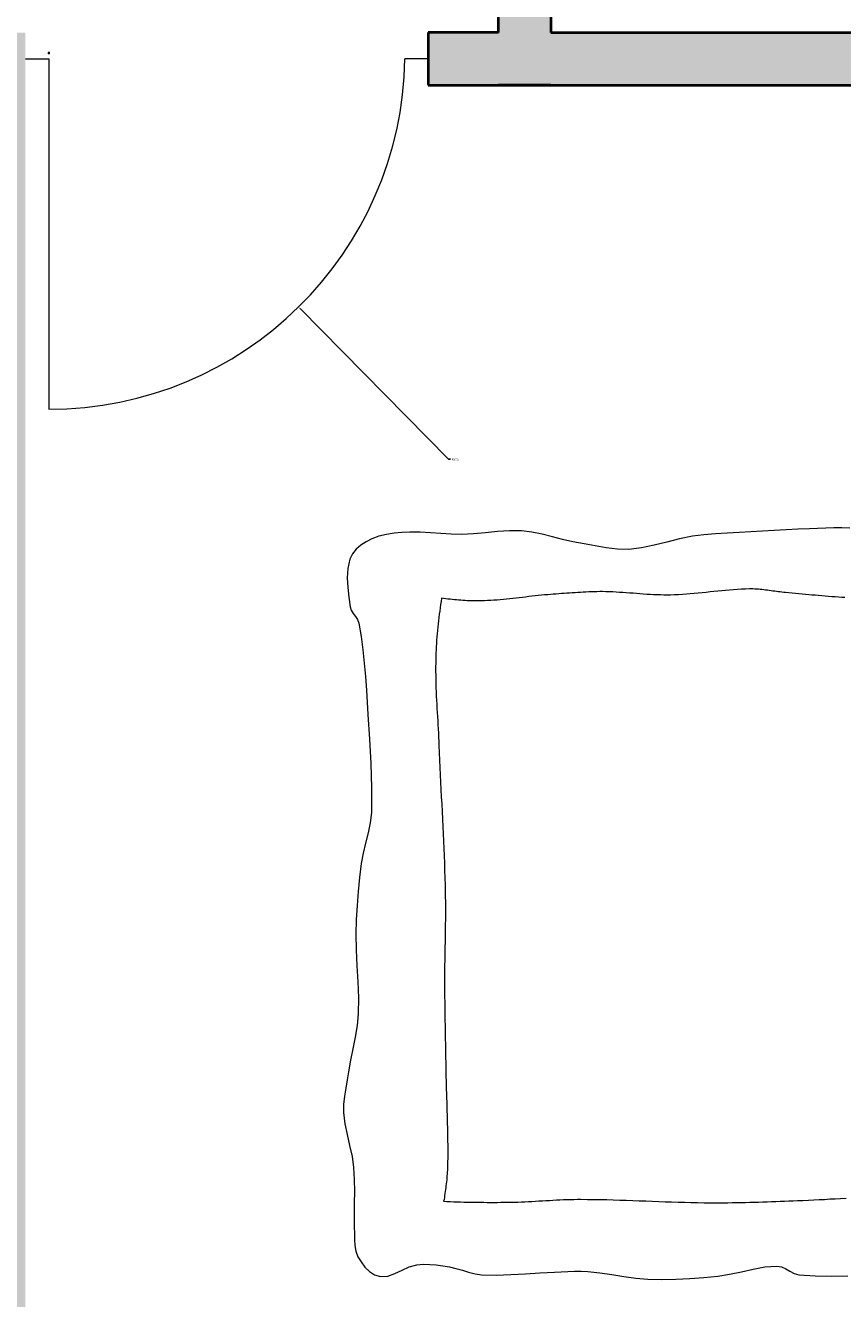
# Model space of a CAD drawing. Units: inches. Extents: x 1441 to 2460, y 1648 to 2683.
# Tile 4 of 35: x 1760 to 1830, y 1866 to 1975. Entities that reach past the tile are written whole.
import ezdxf

# ---------------------------------------------------------------- set-up
doc = ezdxf.new("R2010")
doc.units = ezdxf.units.IN
for name, color, linetype, lineweight in [('A-ANNO-DIMS', 2, 'Continuous', 18), ('A-DOOR', 3, 'Continuous', 20), ('A-FURN', 8, 'Continuous', 15), ('A-WALL', 7, 'Continuous', 40)]:
    doc.layers.add(name, color=color, linetype=linetype, lineweight=lineweight)
doc.layers.add('A-WALL-PATT', color=251, linetype='Continuous', lineweight=13, true_color=0x636466)
doc.styles.get("Standard").update_dxf_attribs({"font": 'arial.ttf'})
doc.dimstyles.get("Standard").update_dxf_attribs({"dimtxt": 0.18, "dimasz": 0.18, "dimexe": 0.18, "dimexo": 0.0625, "dimgap": 0.09, "dimtad": 0, "dimtih": 1, "dimtoh": 1, "dimdec": 4, "dimzin": 0, "dimdsep": 46, "dimtxsty": 'Standard', "dimcen": 0.09, "dimadec": 0, "dimazin": 0, "dimtfac": 1, "dimtdec": 4, "dimtofl": 0, "dimtmove": 0, "dimatfit": 3, "dimfxl": 1, "dimtolj": 1, "dimtzin": 0, "dimarcsym": 0})

# ---------------------------------------------------------------- blocks, each defined once
blk = doc.blocks.new('BED-DOUBLE-PLAN')
for p, q in [((0.03, 43.36), (0, 42.67)), ((0, 42.67), (0, 41.98)), ((5.96, 42.66), (5.93, 42.38)), ((5.97, 42.94), (5.96, 42.66)), ((57.42, 42.57), (57.39, 43.03)), ((57.45, 42.11), (57.42, 42.57)), ((64.07, 41.78), (64.06, 43.17)), ((0, 41.98), (0.02, 41.29)), ((5.87, 41.53), (5.85, 41.24)), ((5.89, 41.81), (5.87, 41.53)), ((5.91, 42.09), (5.89, 41.81)), ((5.93, 42.38), (5.91, 42.09)), ((57.47, 41.65), (57.45, 42.11)), ((57.5, 41.19), (57.47, 41.65)), ((64.05, 40.38), (64.07, 41.78)), ((0.02, 41.29), (0.05, 40.6)), ((0.05, 40.6), (0.08, 39.91)), ((5.77, 40.39), (5.75, 40.11)), ((5.8, 40.68), (5.77, 40.39)), ((5.82, 40.96), (5.8, 40.68)), ((5.85, 41.24), (5.82, 40.96)), ((57.52, 40.73), (57.5, 41.19)), ((57.55, 40.27), (57.52, 40.73)), ((63.96, 38.99), (64.05, 40.38)), ((0.08, 39.91), (0.12, 38.9)), ((5.67, 39.26), (5.65, 38.98)), ((5.7, 39.55), (5.67, 39.26)), ((5.72, 39.83), (5.7, 39.55)), ((5.75, 40.11), (5.72, 39.83)), ((57.57, 39.81), (57.55, 40.27)), ((57.59, 39.34), (57.57, 39.81)), ((57.61, 38.88), (57.59, 39.34)), ((0.12, 38.9), (0.17, 37.89)), ((5.6, 38.41), (5.57, 38.13)), ((5.62, 38.7), (5.6, 38.41)), ((5.65, 38.98), (5.62, 38.7)), ((57.62, 38.51), (57.61, 38.88)), ((57.64, 38.14), (57.62, 38.51)), ((63.45, 37.87), (63.66, 38.23)), ((63.66, 38.23), (63.85, 38.6)), ((63.85, 38.6), (63.96, 38.99)), ((0.17, 37.89), (0.23, 36.88)), ((5.45, 37.07), (5.43, 36.92)), ((5.47, 37.23), (5.45, 37.07)), ((5.49, 37.38), (5.47, 37.23)), ((5.51, 37.54), (5.49, 37.38)), ((5.53, 37.69), (5.51, 37.54)), ((5.54, 37.85), (5.53, 37.69)), ((5.57, 38.13), (5.54, 37.85)), ((57.65, 37.77), (57.64, 38.14)), ((57.67, 37.39), (57.65, 37.77)), ((57.68, 37.02), (57.67, 37.39)), ((63.21, 37.11), (63.27, 37.5)), ((63.29, 36.09), (63.21, 37.11)), ((63.27, 37.5), (63.45, 37.87)), ((0.23, 36.88), (0.29, 35.88)), ((5.3, 35.99), (5.29, 35.83)), ((5.32, 36.14), (5.3, 35.99)), ((5.34, 36.3), (5.32, 36.14)), ((5.37, 36.45), (5.34, 36.3)), ((5.39, 36.61), (5.37, 36.45)), ((5.41, 36.76), (5.39, 36.61)), ((5.43, 36.92), (5.41, 36.76)), ((57.69, 36.65), (57.68, 37.02)), ((57.71, 36.27), (57.69, 36.65)), ((57.72, 35.9), (57.71, 36.27)), ((63.47, 35.08), (63.29, 36.09)), ((0.29, 35.88), (0.35, 34.87)), ((5.24, 35.21), (5.23, 35.06)), ((5.23, 35.06), (5.23, 34.9)), ((5.23, 34.9), (5.23, 34.75)), ((5.26, 35.52), (5.24, 35.37)), ((5.24, 35.37), (5.24, 35.21)), ((5.27, 35.68), (5.26, 35.52)), ((5.29, 35.83), (5.27, 35.68)), ((57.73, 35.53), (57.72, 35.9)), ((57.74, 35.15), (57.73, 35.53)), ((57.75, 34.78), (57.74, 35.15)), ((63.7, 34.07), (63.47, 35.08)), ((0.35, 34.87), (0.4, 33.87)), ((0.4, 33.87), (0.46, 32.86)), ((5.23, 34.75), (5.24, 34.41)), ((5.24, 34.41), (5.25, 34.07)), ((5.25, 34.07), (5.27, 33.73)), ((57.76, 34.41), (57.75, 34.78)), ((57.77, 34.04), (57.76, 34.41)), ((57.78, 33.66), (57.77, 34.04)), ((63.92, 33.06), (63.7, 34.07)), ((0.46, 32.86), (0.52, 31.86)), ((5.27, 33.73), (5.3, 33.4)), ((5.3, 33.4), (5.32, 33.06)), ((5.32, 33.06), (5.35, 32.72)), ((5.35, 32.72), (5.39, 32.39)), ((57.78, 33.29), (57.78, 33.66)), ((57.79, 32.92), (57.78, 33.29)), ((57.79, 32.54), (57.79, 32.92)), ((64.08, 32.05), (63.92, 33.06)), ((0.52, 31.86), (0.6, 30.86)), ((5.39, 32.39), (5.42, 32.05)), ((5.42, 32.05), (5.46, 31.71)), ((5.46, 31.71), (5.49, 31.38)), ((57.79, 32.17), (57.79, 32.54)), ((57.79, 31.8), (57.79, 32.17)), ((57.79, 31.42), (57.79, 31.8)), ((64.19, 30.85), (64.08, 32.05)), ((0.6, 30.86), (0.72, 29.87)), ((5.49, 31.38), (5.53, 31.04)), ((5.53, 31.04), (5.56, 30.7)), ((5.56, 30.7), (5.59, 30.37)), ((57.78, 30.31), (57.79, 30.87)), ((57.79, 30.87), (57.79, 31.42)), ((64.27, 29.65), (64.19, 30.85)), ((0.72, 29.87), (0.93, 28.77)), ((5.59, 30.37), (5.63, 30.03)), ((5.63, 30.03), (5.66, 29.69)), ((5.66, 29.69), (5.68, 29.36)), ((57.75, 29.2), (57.77, 29.76)), ((57.77, 29.76), (57.78, 30.31)), ((64.33, 28.45), (64.27, 29.65)), ((0.93, 28.77), (1.21, 27.69)), ((5.68, 29.36), (5.71, 29.02)), ((5.71, 29.02), (5.73, 28.68)), ((5.73, 28.68), (5.74, 28.34)), ((57.72, 28.09), (57.74, 28.65)), ((57.74, 28.65), (57.75, 29.2)), ((64.35, 27.25), (64.33, 28.45)), ((1.21, 27.69), (1.49, 26.61)), ((5.74, 28.34), (5.75, 28.01)), ((5.75, 27.42), (5.74, 27.13)), ((5.75, 28.01), (5.75, 27.71)), ((5.75, 27.71), (5.75, 27.42)), ((57.68, 26.99), (57.7, 27.54)), ((57.7, 27.54), (57.72, 28.09)), ((1.49, 26.61), (1.72, 25.52)), ((5.7, 26.26), (5.69, 25.96)), ((5.72, 26.55), (5.7, 26.26)), ((5.73, 26.84), (5.72, 26.55)), ((5.74, 27.13), (5.73, 26.84)), ((57.64, 25.88), (57.66, 26.43)), ((57.66, 26.43), (57.68, 26.99)), ((64.33, 26.05), (64.35, 27.25)), ((1.72, 25.52), (1.85, 24.42)), ((5.62, 25.09), (5.6, 24.8)), ((5.64, 25.38), (5.62, 25.09)), ((5.67, 25.67), (5.64, 25.38)), ((5.69, 25.96), (5.67, 25.67)), ((57.59, 24.77), (57.62, 25.32)), ((57.62, 25.32), (57.64, 25.88)), ((64.25, 25.02), (64.33, 26.05)), ((1.85, 24.42), (1.83, 23.46)), ((5.56, 24.21), (5.54, 23.92)), ((5.58, 24.51), (5.56, 24.21)), ((5.6, 24.8), (5.58, 24.51)), ((57.56, 23.66), (57.57, 24.21)), ((57.57, 24.21), (57.59, 24.77)), ((63.94, 22.97), (64.11, 23.99)), ((64.11, 23.99), (64.25, 25.02)), ((1.83, 23.46), (1.72, 22.5)), ((5.49, 23.05), (5.47, 22.75)), ((5.5, 23.34), (5.49, 23.05)), ((5.52, 23.63), (5.5, 23.34)), ((5.54, 23.92), (5.52, 23.63)), ((57.52, 22.55), (57.54, 23.1)), ((57.54, 23.1), (57.56, 23.66)), ((63.78, 21.94), (63.94, 22.97)), ((1.72, 22.5), (1.55, 21.54)), ((5.47, 22.46), (5.46, 22.17)), ((5.46, 22.17), (5.46, 21.94)), ((5.46, 21.94), (5.47, 21.7)), ((5.47, 22.75), (5.47, 22.46)), ((57.5, 21.44), (57.51, 21.99)), ((57.51, 21.99), (57.52, 22.55)), ((63.67, 20.91), (63.78, 21.94)), ((1.55, 21.54), (1.36, 20.59)), ((5.47, 21.7), (5.47, 21.47)), ((5.47, 21.47), (5.48, 21.23)), ((5.48, 21.23), (5.49, 21)), ((5.49, 21), (5.5, 20.76)), ((5.5, 20.76), (5.51, 20.53)), ((57.49, 20.33), (57.5, 20.88)), ((57.5, 20.88), (57.5, 21.44)), ((63.65, 20.35), (63.67, 20.91)), ((1.18, 19.64), (1, 18.76)), ((1.36, 20.59), (1.18, 19.64)), ((5.51, 20.53), (5.52, 20.29)), ((5.52, 20.29), (5.53, 20.06)), ((5.53, 20.06), (5.55, 19.83)), ((5.55, 19.83), (5.56, 19.59)), ((57.49, 20.03), (57.49, 20.33)), ((57.5, 19.73), (57.49, 20.03)), ((57.5, 19.43), (57.5, 19.73)), ((63.66, 19.78), (63.65, 20.35)), ((63.68, 19.21), (63.66, 19.78)), ((1, 18.76), (0.77, 17.89)), ((5.56, 19.59), (5.58, 19.36)), ((5.58, 19.36), (5.59, 19.12)), ((5.59, 19.12), (5.61, 18.89)), ((5.61, 18.89), (5.63, 18.66)), ((5.63, 18.66), (5.65, 18.42)), ((57.51, 19.13), (57.5, 19.43)), ((57.52, 18.83), (57.51, 19.13)), ((57.54, 18.53), (57.52, 18.83)), ((63.71, 18.64), (63.68, 19.21)), ((63.74, 18.07), (63.71, 18.64)), ((0.77, 17.89), (0.55, 17.01)), ((5.65, 18.42), (5.67, 18.19)), ((5.67, 18.19), (5.68, 17.95)), ((5.68, 17.95), (5.7, 17.72)), ((5.7, 17.72), (5.72, 17.49)), ((5.72, 17.49), (5.74, 17.21)), ((57.55, 18.23), (57.54, 18.53)), ((57.57, 17.93), (57.55, 18.23)), ((57.59, 17.63), (57.57, 17.93)), ((57.6, 17.33), (57.59, 17.63)), ((63.8, 16.82), (63.74, 18.07)), ((0.55, 17.01), (0.37, 16.13)), ((5.74, 17.21), (5.77, 16.94)), ((5.77, 16.94), (5.79, 16.67)), ((5.79, 16.67), (5.82, 16.4)), ((5.82, 16.4), (5.85, 16.13)), ((57.62, 17.03), (57.6, 17.33)), ((57.64, 16.73), (57.62, 17.03)), ((57.66, 16.43), (57.64, 16.73)), ((57.68, 16.13), (57.66, 16.43)), ((63.88, 15.57), (63.8, 16.82)), ((0.37, 16.13), (0.26, 15.25)), ((5.85, 16.13), (5.88, 15.86)), ((5.88, 15.86), (5.92, 15.59)), ((5.92, 15.59), (5.95, 15.32)), ((5.95, 15.32), (5.98, 15.04)), ((57.69, 15.83), (57.68, 16.13)), ((57.71, 15.53), (57.69, 15.83)), ((57.72, 15.23), (57.71, 15.53)), ((63.95, 14.32), (63.88, 15.57)), ((0.26, 15.25), (0.24, 14.22)), ((0.24, 14.22), (0.31, 13.19)), ((5.98, 15.04), (6.01, 14.77)), ((6.01, 14.77), (6.04, 14.5)), ((6.04, 14.5), (6.07, 14.23)), ((6.07, 14.23), (6.1, 13.96)), ((57.73, 14.93), (57.72, 15.23)), ((57.74, 14.63), (57.73, 14.93)), ((57.74, 14.33), (57.74, 14.63)), ((57.75, 14.04), (57.74, 14.33)), ((63.99, 13.07), (63.95, 14.32)), ((0.31, 13.19), (0.41, 12.16)), ((6.1, 13.96), (6.13, 13.69)), ((6.13, 13.69), (6.16, 13.42)), ((6.16, 13.42), (6.18, 13.15)), ((6.18, 13.15), (6.2, 12.88)), ((57.75, 13.75), (57.75, 14.04)), ((57.75, 13.46), (57.75, 13.75)), ((57.76, 13.17), (57.75, 13.46)), ((57.76, 12.89), (57.76, 13.17)), ((0.41, 12.16), (0.51, 11.13)), ((6.2, 12.88), (6.22, 12.6)), ((6.22, 12.6), (6.23, 12.33)), ((6.23, 12.33), (6.24, 12.06)), ((6.24, 12.06), (6.25, 11.88)), ((57.75, 12.02), (57.76, 12.31)), ((57.75, 11.73), (57.75, 12.02)), ((57.76, 12.6), (57.76, 12.89)), ((57.76, 12.31), (57.76, 12.6)), ((63.96, 11.82), (63.99, 13.07)), ((0.51, 11.13), (0.56, 10.1)), ((6.25, 10.96), (6.24, 10.77)), ((6.25, 11.88), (6.25, 11.69)), ((6.25, 11.69), (6.25, 11.51)), ((6.25, 11.51), (6.25, 11.32)), ((6.25, 11.32), (6.25, 11.14)), ((6.25, 11.14), (6.25, 10.96)), ((57.74, 11.16), (57.75, 11.45)), ((57.74, 10.87), (57.74, 11.16)), ((57.75, 11.45), (57.75, 11.73)), ((63.75, 10.71), (63.89, 11.26)), ((63.89, 11.26), (63.96, 11.82)), ((0.56, 10.1), (0.54, 9.21)), ((6.19, 9.85), (6.17, 9.67)), ((6.2, 10.04), (6.19, 9.85)), ((6.22, 10.22), (6.2, 10.04)), ((6.23, 10.4), (6.22, 10.22)), ((6.24, 10.59), (6.23, 10.4)), ((6.24, 10.77), (6.24, 10.59)), ((57.71, 9.72), (57.72, 10.01)), ((57.72, 10.01), (57.73, 10.29)), ((57.73, 10.58), (57.74, 10.87)), ((57.73, 10.29), (57.73, 10.58)), ((63.41, 9.62), (63.57, 10.17)), ((63.57, 10.17), (63.75, 10.71)), ((0.54, 9.21), (0.48, 8.33)), ((6.07, 8.76), (6.04, 8.57)), ((6.09, 8.94), (6.07, 8.76)), ((6.11, 9.12), (6.09, 8.94)), ((6.14, 9.3), (6.11, 9.12)), ((6.16, 9.49), (6.14, 9.3)), ((6.17, 9.67), (6.16, 9.49)), ((44.18, 8.72), (44.58, 8.72)), ((44.58, 8.72), (44.98, 8.73)), ((44.98, 8.73), (45.38, 8.74)), ((45.38, 8.74), (45.77, 8.75)), ((45.77, 8.75), (46.17, 8.75)), ((46.17, 8.75), (46.57, 8.76)), ((46.57, 8.76), (46.97, 8.77)), ((46.97, 8.77), (47.34, 8.78)), ((47.34, 8.78), (47.7, 8.78)), ((47.7, 8.78), (48.07, 8.79)), ((48.07, 8.79), (48.44, 8.8)), ((48.44, 8.8), (48.81, 8.82)), ((48.81, 8.82), (49.17, 8.83)), ((49.17, 8.83), (49.54, 8.84)), ((49.54, 8.84), (49.91, 8.85)), ((49.91, 8.85), (50.28, 8.86)), ((50.28, 8.86), (50.65, 8.87)), ((50.65, 8.87), (51.01, 8.88)), ((51.01, 8.88), (51.38, 8.89)), ((51.38, 8.89), (51.75, 8.9)), ((51.75, 8.9), (52.12, 8.91)), ((52.12, 8.91), (52.48, 8.91)), ((52.48, 8.91), (52.85, 8.92)), ((52.85, 8.92), (53.22, 8.92)), ((53.22, 8.92), (53.59, 8.92)), ((53.59, 8.92), (53.95, 8.92)), ((53.95, 8.92), (54.32, 8.91)), ((54.32, 8.91), (54.49, 8.91)), ((54.49, 8.91), (54.66, 8.9)), ((54.66, 8.9), (54.83, 8.9)), ((54.83, 8.9), (55, 8.89)), ((55, 8.89), (55.16, 8.88)), ((55.16, 8.88), (55.33, 8.87)), ((55.33, 8.87), (55.5, 8.85)), ((55.5, 8.85), (55.67, 8.84)), ((55.67, 8.84), (55.84, 8.83)), ((55.84, 8.83), (56, 8.81)), ((56, 8.81), (56.17, 8.79)), ((56.17, 8.79), (56.34, 8.77)), ((56.34, 8.77), (56.51, 8.75)), ((56.51, 8.75), (56.67, 8.73)), ((56.67, 8.73), (56.84, 8.71)), ((57.67, 8.57), (57.68, 8.85)), ((57.68, 8.85), (57.69, 9.14)), ((57.69, 9.14), (57.7, 9.43)), ((57.7, 9.43), (57.71, 9.72)), ((63.2, 8.51), (63.28, 9.07)), ((63.28, 9.07), (63.41, 9.62)), ((0.48, 8.33), (0.41, 7.44)), ((6.04, 8.57), (6.01, 8.39)), ((6.01, 8.39), (6.29, 8.35)), ((6.29, 8.35), (6.56, 8.31)), ((6.56, 8.31), (6.84, 8.27)), ((6.84, 8.27), (7.12, 8.23)), ((7.12, 8.23), (7.39, 8.19)), ((7.39, 8.19), (7.67, 8.16)), ((7.67, 8.16), (7.95, 8.12)), ((7.95, 8.12), (8.23, 8.09)), ((8.23, 8.09), (8.5, 8.07)), ((8.5, 8.07), (8.78, 8.04)), ((8.78, 8.04), (9.06, 8.02)), ((9.06, 8.02), (9.34, 7.99)), ((9.34, 7.99), (9.62, 7.97)), ((9.62, 7.97), (9.9, 7.95)), ((9.9, 7.95), (10.18, 7.94)), ((10.18, 7.94), (10.45, 7.92)), ((10.45, 7.92), (10.73, 7.91)), ((10.73, 7.91), (11.01, 7.9)), ((11.01, 7.9), (11.29, 7.89)), ((11.29, 7.89), (11.57, 7.89)), ((11.57, 7.89), (11.92, 7.88)), ((11.92, 7.88), (12.28, 7.88)), ((12.28, 7.88), (12.63, 7.89)), ((12.63, 7.89), (12.98, 7.89)), ((12.98, 7.89), (13.34, 7.9)), ((13.34, 7.9), (13.69, 7.91)), ((13.69, 7.91), (14.04, 7.92)), ((14.04, 7.92), (14.4, 7.94)), ((14.4, 7.94), (14.75, 7.96)), ((14.75, 7.96), (15.1, 7.98)), ((15.1, 7.98), (15.46, 7.99)), ((15.46, 7.99), (15.81, 8.01)), ((15.81, 8.01), (16.16, 8.04)), ((16.16, 8.04), (16.52, 8.06)), ((16.52, 8.06), (16.87, 8.08)), ((16.87, 8.08), (17.22, 8.1)), ((17.22, 8.1), (17.58, 8.12)), ((17.58, 8.12), (17.93, 8.13)), ((17.93, 8.13), (18.28, 8.15)), ((18.28, 8.15), (18.64, 8.17)), ((18.64, 8.17), (19.27, 8.19)), ((19.27, 8.19), (19.9, 8.22)), ((19.9, 8.22), (20.52, 8.25)), ((20.52, 8.25), (21.15, 8.28)), ((21.15, 8.28), (21.78, 8.31)), ((21.78, 8.31), (22.41, 8.34)), ((22.41, 8.34), (23.04, 8.37)), ((23.04, 8.37), (23.67, 8.4)), ((23.67, 8.4), (24.3, 8.43)), ((24.3, 8.43), (24.93, 8.46)), ((24.93, 8.46), (25.56, 8.49)), ((25.56, 8.49), (26.19, 8.52)), ((26.19, 8.52), (26.82, 8.55)), ((26.82, 8.55), (27.45, 8.58)), ((27.45, 8.58), (28.08, 8.6)), ((28.08, 8.6), (28.71, 8.63)), ((28.71, 8.63), (29.33, 8.65)), ((29.33, 8.65), (29.96, 8.67)), ((29.96, 8.67), (30.59, 8.69)), ((30.59, 8.69), (31.22, 8.7)), ((31.22, 8.7), (31.61, 8.71)), ((31.61, 8.71), (32, 8.72)), ((32, 8.72), (32.39, 8.72)), ((32.39, 8.72), (32.78, 8.72)), ((32.78, 8.72), (33.17, 8.72)), ((33.17, 8.72), (33.56, 8.72)), ((33.56, 8.72), (33.95, 8.71)), ((33.95, 8.71), (34.34, 8.71)), ((34.34, 8.71), (34.73, 8.7)), ((34.73, 8.7), (35.12, 8.69)), ((35.12, 8.69), (35.51, 8.69)), ((35.51, 8.69), (35.89, 8.68)), ((35.89, 8.68), (36.28, 8.67)), ((36.28, 8.67), (36.67, 8.67)), ((36.67, 8.67), (37.06, 8.66)), ((37.06, 8.66), (37.45, 8.65)), ((37.45, 8.65), (37.84, 8.65)), ((37.84, 8.65), (38.23, 8.65)), ((38.23, 8.65), (38.62, 8.64)), ((38.62, 8.64), (39.01, 8.65)), ((39.01, 8.65), (39.41, 8.65)), ((39.41, 8.65), (39.81, 8.65)), ((39.81, 8.65), (40.2, 8.65)), ((40.2, 8.65), (40.6, 8.66)), ((40.6, 8.66), (41, 8.66)), ((41, 8.66), (41.4, 8.67)), ((41.4, 8.67), (41.8, 8.67)), ((41.8, 8.67), (42.19, 8.68)), ((42.19, 8.68), (42.59, 8.69)), ((42.59, 8.69), (42.99, 8.69)), ((42.99, 8.69), (43.39, 8.7)), ((43.39, 8.7), (43.78, 8.71)), ((43.78, 8.71), (44.18, 8.72)), ((56.84, 8.71), (57.01, 8.68)), ((57.01, 8.68), (57.17, 8.65)), ((57.17, 8.65), (57.34, 8.63)), ((57.34, 8.63), (57.51, 8.6)), ((57.51, 8.6), (57.67, 8.57)), ((63.07, 7.38), (63.12, 7.94)), ((63.12, 7.94), (63.2, 8.51)), ((0.41, 7.44), (0.36, 6.56)), ((0.36, 6.56), (0.37, 5.67)), ((63.06, 6.82), (63.07, 7.38)), ((63.1, 6.26), (63.06, 6.82)), ((0.37, 5.67), (0.4, 5)), ((63.28, 5.62), (63.1, 6.26)), ((63.56, 5.01), (63.28, 5.62)), ((0.4, 5), (0.46, 4.34)), ((63.86, 4.4), (63.56, 5.01)), ((64.07, 3.78), (63.86, 4.4)), ((0.46, 4.34), (0.56, 3.68)), ((0.56, 3.68), (0.71, 3.03)), ((64.1, 3.15), (64.07, 3.78)), ((0.71, 3.03), (0.94, 2.41)), ((0.94, 2.41), (1.18, 1.94)), ((15.99, 2.09), (18.08, 2.23)), ((18.08, 2.23), (20.17, 2.34)), ((20.17, 2.34), (22.27, 2.4)), ((22.27, 2.4), (24.37, 2.38)), ((24.37, 2.38), (25.25, 2.29)), ((25.25, 2.29), (26.12, 2.11)), ((63.3, 1.83), (63.67, 2.22)), ((63.67, 2.22), (63.96, 2.66)), ((63.96, 2.66), (64.1, 3.15)), ((1.18, 1.94), (1.48, 1.49)), ((1.48, 1.49), (1.83, 1.09)), ((7.58, 1.03), (7.85, 1.2)), ((7.85, 1.2), (8.15, 1.31)), ((8.15, 1.31), (9.29, 1.5)), ((9.29, 1.5), (10.43, 1.66)), ((10.43, 1.66), (11.58, 1.77)), ((11.58, 1.77), (12.74, 1.87)), ((12.74, 1.87), (13.89, 1.95)), ((13.89, 1.95), (15.99, 2.09)), ((26.12, 2.11), (26.99, 1.88)), ((26.99, 1.88), (27.86, 1.67)), ((27.86, 1.67), (28.74, 1.51)), ((28.74, 1.51), (29.94, 1.37)), ((29.94, 1.37), (31.14, 1.25)), ((31.14, 1.25), (32.35, 1.16)), ((32.35, 1.16), (33.55, 1.09)), ((36.13, 1.07), (37.5, 1.14)), ((37.5, 1.14), (38.87, 1.22)), ((38.87, 1.22), (40.25, 1.28)), ((40.25, 1.28), (41.62, 1.25)), ((41.62, 1.25), (42.61, 1.16)), ((42.61, 1.16), (43.61, 0.99)), ((61.94, 1.05), (62.41, 1.23)), ((62.41, 1.23), (62.86, 1.5)), ((62.86, 1.5), (63.3, 1.83)), ((1.83, 1.09), (2.23, 0.76)), ((2.23, 0.76), (2.69, 0.54)), ((2.69, 0.54), (3.48, 0.36)), ((3.48, 0.36), (4.29, 0.31)), ((4.29, 0.31), (5.11, 0.35)), ((5.11, 0.35), (5.93, 0.45)), ((5.93, 0.45), (6.75, 0.56)), ((6.75, 0.56), (7.04, 0.66)), ((7.04, 0.66), (7.32, 0.83)), ((7.32, 0.83), (7.58, 1.03)), ((33.55, 1.09), (34.76, 1.05)), ((34.76, 1.05), (36.13, 1.07)), ((43.61, 0.99), (44.6, 0.79)), ((44.6, 0.79), (45.58, 0.59)), ((45.58, 0.59), (46.58, 0.41)), ((46.58, 0.41), (47.27, 0.3)), ((47.27, 0.3), (47.97, 0.18)), ((47.97, 0.18), (48.67, 0.07)), ((48.67, 0.07), (49.37, 0)), ((49.37, 0), (50.07, 0)), ((50.07, 0), (51.02, 0.11)), ((51.02, 0.11), (51.96, 0.3)), ((51.96, 0.3), (52.89, 0.52)), ((52.89, 0.52), (53.83, 0.73)), ((53.83, 0.73), (54.78, 0.86)), ((54.78, 0.86), (55.8, 0.92)), ((55.8, 0.92), (56.82, 0.93)), ((56.82, 0.93), (57.84, 0.91)), ((57.84, 0.91), (58.87, 0.9)), ((58.87, 0.9), (59.89, 0.92)), ((59.89, 0.92), (60.41, 0.93)), ((60.41, 0.93), (60.93, 0.93)), ((60.93, 0.93), (61.44, 0.96)), ((61.44, 0.96), (61.94, 1.05))]:
    blk.add_line(p, q)
blk = doc.blocks.new('DOOR-BED3-30')
for p, q in [((0, 30.01), (2, 30.01)), ((2, 30.01), (2, 0.01)), ((34.49, 30.01), (32.49, 30.01))]:
    blk.add_line(p, q)
blk.add_arc((2, 30.51), 30.5, 270, 359.0598)
blk = doc.blocks.new('*D67')
at = {"layer": 'A-ANNO-DIMS', "color": 0, "lineweight": -2, "transparency": 16777216}
for p, q in [((1889.45, 2298.7), (1916.22, 2298.7)), ((1916.04, 2298.52), (1916.04, 2055.94)), ((1916.04, 1813), (1916.04, 2055.57)), ((1758.22, 1812.82), (1916.22, 1812.82))]:
    blk.add_line(p, q, dxfattribs=at)
at = {"layer": 'A-ANNO-DIMS', "color": 0, "transparency": 16777216}
for points in [[(1916.01, 2298.52), (1916.07, 2298.52), (1916.04, 2298.7)], [(1916.01, 1813), (1916.07, 1813), (1916.04, 1812.82)]]:
    blk.add_solid(points, dxfattribs=at)
at = {"layer": 'Defpoints', "color": 0, "transparency": 16777216}
for p in [(1889.39, 2298.7), (1916.04, 2298.7), (1758.16, 1812.82)]:
    blk.add_point(p, dxfattribs=at)
at = {"layer": 'A-ANNO-DIMS', "color": 0, "transparency": 16777216, "insert": (1916.04, 2055.76), "char_height": 0.18, "attachment_point": 5}
blk.add_mtext('\\A1;485.9', dxfattribs=at)
blk = doc.blocks.new('*D131')
at = {"layer": 'A-ANNO-DIMS', "color": 0, "lineweight": -2, "transparency": 16777216}
for p, q in [((1762.3, 1972.95), (1762.48, 1972.95)), ((1762.39, 1972.86), (1762.39, 1973.04)), ((1796.61, 1938.16), (1783.9, 1951.07)), ((1796.79, 1938.16), (1796.61, 1938.16))]:
    blk.add_line(p, q, dxfattribs=at)
at = {"layer": 'A-ANNO-DIMS', "color": 0, "transparency": 16777216}
blk.add_solid([(1783.92, 1951.09), (1783.88, 1951.05), (1783.77, 1951.2)], dxfattribs=at)
at = {"layer": 'Defpoints', "color": 0, "transparency": 16777216}
for p in [(1762.39, 1972.95), (1783.77, 1951.2)]:
    blk.add_point(p, dxfattribs=at)
at = {"layer": 'A-ANNO-DIMS', "color": 0, "transparency": 16777216, "insert": (1797.2, 1938.16), "char_height": 0.18, "attachment_point": 5}
blk.add_mtext('\\A1;R30.5', dxfattribs=at)

msp = doc.modelspace()

# ---------------------------------------------------------------- hatches: boundary and pattern name
at = {"layer": 'A-WALL-PATT'}
h = msp.add_hatch(color=256, dxfattribs=at)
h.dxf.hatch_style = 1
h.paths.add_polyline_path([(1627.5085, 2298.6952), (1568.8859, 2298.6952), (1568.8859, 2246.9605), (1577.8859, 2246.9605), (1577.8859, 2289.6952), (1627.5085, 2289.6952), (1627.5085, 2294.1952)])
h.paths.add_polyline_path([(1675.5777, 2298.6952), (1651.5085, 2298.6952), (1651.5085, 2289.6952), (1675.5777, 2289.6952), (1675.5777, 2294.1952)])
h.paths.add_polyline_path([(1667.3859, 2289.6952), (1662.8859, 2289.6952), (1662.8859, 2233.0622), (1667.3859, 2233.0622)])
h.paths.add_polyline_path([(1715.8721, 2294.3362), (1715.8721, 2295.2788), (1715.8721, 2298.6952), (1699.5777, 2298.6952), (1699.5777, 2289.6952), (1715.8721, 2289.6952)])
h.paths.add_polyline_path([(1707.8859, 2289.6952), (1703.3859, 2289.6952), (1703.3859, 2199.6952), (1707.8859, 2199.6952)])
h.paths.add_polyline_path([(1760.3859, 2204.637), (1755.8859, 2204.637), (1755.8859, 2199.6952), (1667.3859, 2199.6952), (1667.3859, 2204.637), (1662.8859, 2204.637), (1662.8859, 2195.1952), (1760.3859, 2195.1952)])
h.paths.add_polyline_path([(1760.3859, 2289.6952), (1755.8859, 2289.6952), (1755.8859, 2233.0622), (1760.3859, 2233.0622)])
h.paths.add_polyline_path([(1889.3859, 2298.6952), (1739.8721, 2298.6952), (1739.8721, 2289.6952), (1880.3859, 2289.6952), (1880.3859, 2250.8051), (1889.3859, 2250.8051)])
h.paths.add_polyline_path([(1889.3859, 2202.8051), (1880.3859, 2202.8051), (1880.3859, 2157.6952), (1747.948, 2157.6952), (1747.948, 2153.1952), (1755.8859, 2153.1952), (1755.8859, 2058.005), (1760.3859, 2058.005), (1760.3859, 2153.1952), (1880.3859, 2153.1952), (1880.3859, 2124.108), (1889.3859, 2124.108)])
h.paths.add_polyline_path([(1889.3859, 1984.8305), (1880.3859, 1984.8305), (1880.3859, 1834.1952), (1889.3859, 1834.1952)])
h.paths.add_polyline_path([(1889.3859, 2076.108), (1880.3859, 2076.108), (1880.3859, 2008.8305), (1889.3859, 2008.8305)])
h.paths.add_polyline_path([(1880.3859, 2027.1952), (1800.8859, 2027.1952), (1800.8859, 2000.9452), (1805.3859, 2000.9452), (1805.3859, 2022.6952), (1880.3859, 2022.6952)])
h.paths.add_polyline_path([(1800.8859, 2027.1952), (1760.3859, 2027.1952), (1760.3859, 2030.7912), (1755.8859, 2030.7912), (1755.8859, 2022.6952), (1800.8859, 2022.6952)])
h.paths.add_polyline_path([(1880.3859, 1974.6952), (1805.3859, 1974.6952), (1805.3859, 1978.7973), (1800.8859, 1978.7973), (1800.8859, 1974.6952), (1794.8823, 1974.6952), (1794.8823, 1970.1952), (1800.8859, 1970.1952), (1805.3859, 1970.1952), (1880.3859, 1970.1952)])
h.paths.add_polyline_path([(1760.3859, 1974.6952), (1755.8859, 1974.6952), (1755.8859, 1925.6952), (1751.8616, 1925.6952), (1751.8616, 1921.1952), (1760.3859, 1921.1952)])
h.paths.add_polyline_path([(1760.3859, 1921.1952), (1755.8859, 1921.1952), (1755.8859, 1843.1952), (1760.3859, 1843.1952)])
h.paths.add_polyline_path([(1799.1136, 1838.6952), (1799.1136, 1843.1952), (1760.3859, 1843.1952), (1751.8944, 1843.1952), (1751.8944, 1834.1952), (1758.1615, 1834.1952), (1799.1136, 1834.1952)])
h.paths.add_polyline_path([(1880.3859, 1843.1952), (1859.1136, 1843.1952), (1859.1136, 1834.1952), (1880.3859, 1834.1952)])
h.paths.add_polyline_path([(1577.8859, 1857.7914), (1568.8859, 1857.7914), (1568.8859, 1834.1952), (1695.0034, 1834.1952), (1695.0034, 1838.6952), (1695.0034, 1843.1952), (1577.8859, 1843.1952)])
h.paths.add_polyline_path([(1577.8859, 1959.2399), (1573.3859, 1959.2399), (1568.8859, 1959.2399), (1568.8859, 1905.7914), (1577.8859, 1905.7914), (1577.8859, 1921.1952), (1703.3859, 1921.1952), (1707.8859, 1921.1952), (1715.1501, 1921.1952), (1715.1501, 1925.6952), (1707.8859, 1925.6952), (1703.3859, 1925.6952), (1577.8859, 1925.6952)])
h.paths.add_polyline_path([(1577.8859, 2106.6907), (1568.8859, 2106.6907), (1568.8859, 2019.2399), (1577.8859, 2019.2399)])
h.paths.add_polyline_path([(1707.8859, 2051.6952), (1703.3859, 2051.6952), (1703.3859, 2048.6952), (1703.3859, 1925.6952), (1707.8859, 1925.6952)])
h.paths.add_polyline_path([(1703.3859, 2051.6952), (1676.3859, 2051.6952), (1676.3859, 2048.6952), (1703.3859, 2048.6952)])
h.paths.add_polyline_path([(1703.3859, 2102.6952), (1676.3859, 2102.6952), (1676.3859, 2099.6952), (1685.3859, 2099.6952), (1703.3859, 2099.6952)])
h.paths.add_polyline_path([(1707.8859, 2153.1952), (1710.5611, 2153.1952), (1710.5611, 2157.6952), (1707.8859, 2157.6952), (1707.8859, 2195.1952), (1703.3859, 2195.1952), (1703.3859, 2099.6952), (1707.8859, 2099.6952)])
h.paths.add_polyline_path([(1577.8859, 2198.9605), (1568.8859, 2198.9605), (1568.8859, 2166.6907), (1577.8859, 2166.6907)])

# ---------------------------------------------------------------- linework, layer by layer
at = {"layer": 'A-WALL'}
for p, q in [((1800.8859, 1974.6952), (1800.8859, 1978.7973)), ((1805.3859, 1978.7973), (1805.3859, 1974.6952)), ((1800.8859, 1974.6952), (1794.8823, 1974.6952)), ((1794.8823, 1974.6952), (1794.8823, 1974.6952)), ((1794.8823, 1974.6952), (1794.8823, 1970.1952)), ((1805.3859, 1974.6952), (1880.3859, 1974.6952)), ((1794.8823, 1970.1952), (1800.8859, 1970.1952)), ((1800.8859, 1970.1952), (1880.3859, 1970.1952)), ((1805.3859, 1970.1952), (1800.8859, 1970.1952))]:
    msp.add_line(p, q, dxfattribs=at)

# ---------------------------------------------------------------- block references
at = {"layer": 'A-DOOR'}
msp.add_blockref('DOOR-BED3-30', (1760.39, 1942.44), dxfattribs=at)
at = {"layer": 'A-FURN', "rotation": 270}
msp.add_blockref('BED-DOUBLE-PLAN', (1787.6309, 1932.2861), dxfattribs=at)

# ---------------------------------------------------------------- dimensions: what is measured, and where the dimension line sits
at = {"layer": 'A-ANNO-DIMS'}
dim = msp.add_linear_dim(base=(1916.0359, 2298.6952), p1=(1758.1615, 1812.8171), p2=(1889.3859, 2298.6952), angle=90, dimstyle='Standard', override={"dimdec": 1, "dimlfac": 1, "dimrnd": 0, "dimzin": 0, "dimdsep": 46, "dimlunit": 2}, dxfattribs=at)
dim.commit()
dim.dimension.update_dxf_attribs({"geometry": '*D67', "text_midpoint": (1916.0359, 2055.7561)})
dim = msp.add_radius_dim(center=(1762.3859, 1972.9457), mpoint=(1783.775, 1951.202), dimstyle='Standard', override={"dimdec": 1, "dimlfac": 1, "dimrnd": 0, "dimzin": 0, "dimdsep": 46, "dimlunit": 2}, dxfattribs=at)
dim.commit()
dim.dimension.update_dxf_attribs({"geometry": '*D131', "text_midpoint": (1797.199, 1938.1558), "dimtype": 164})

doc.saveas('drawing.dxf')
